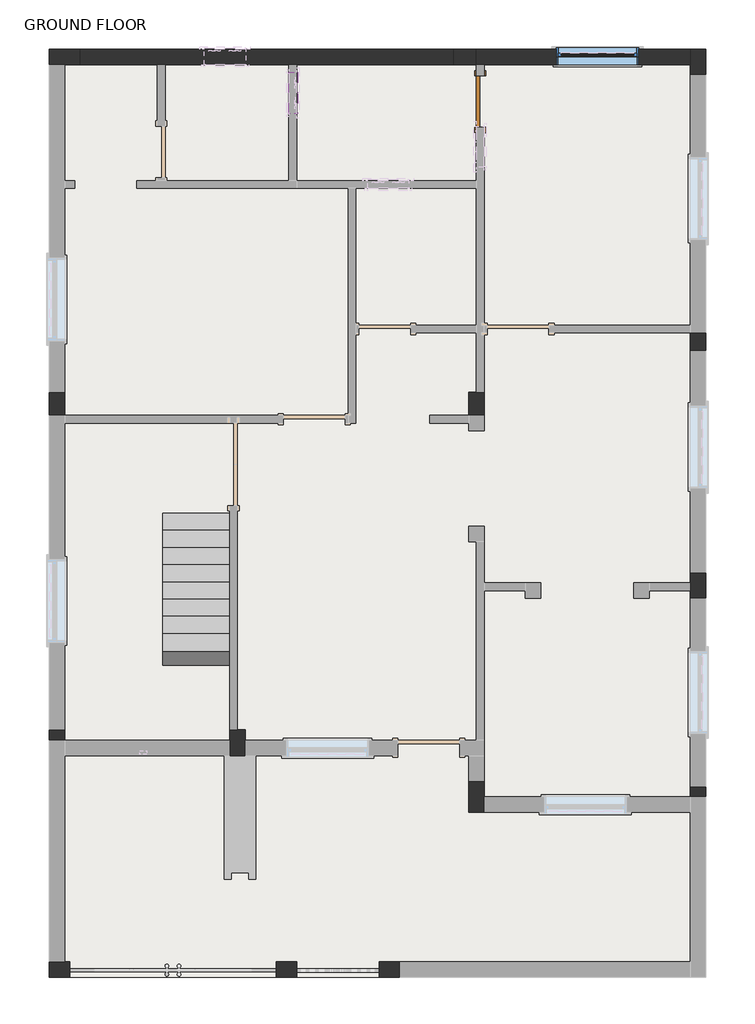
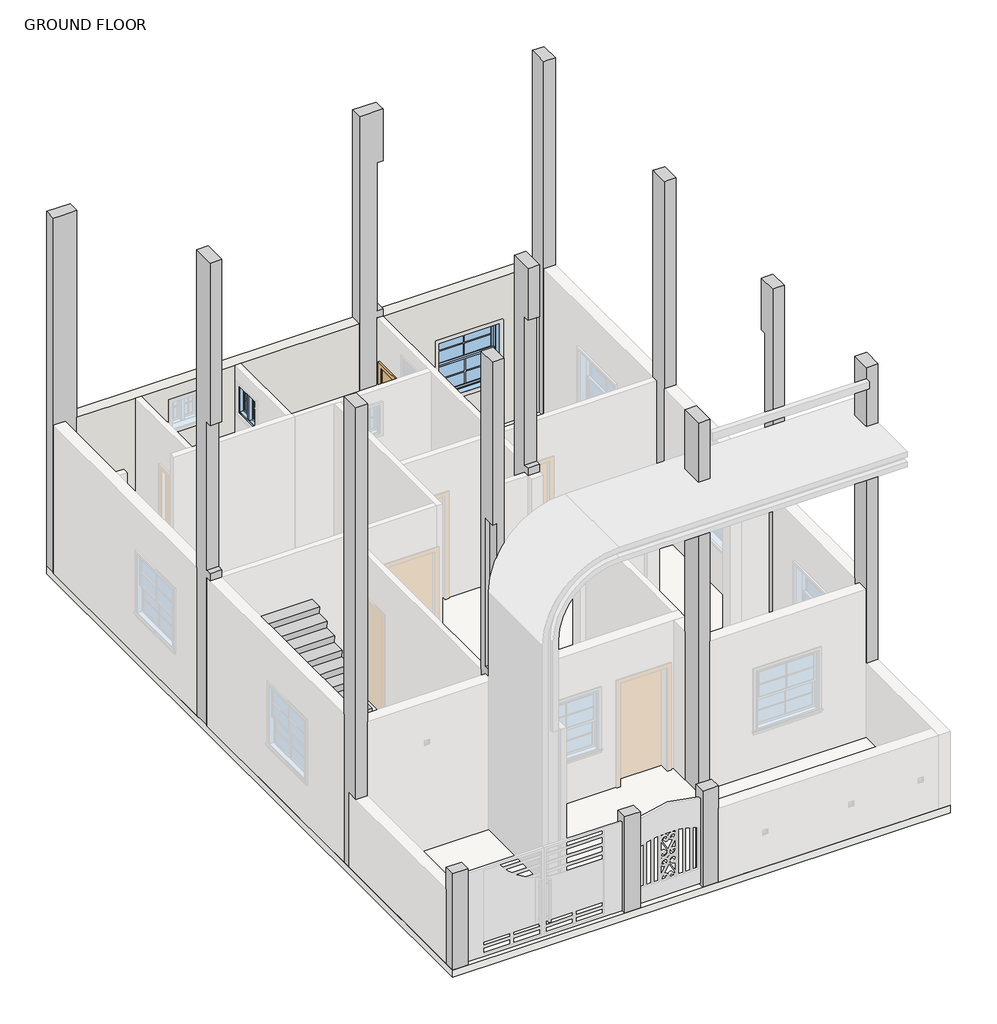
# One storey, part 2 of 3: 14 columns, 2 walls, 2 windows, 1 door, 1 slab, 1 stair flight.
"""IFC4 building model written with IfcOpenShell, lengths in millimetres."""

from ifc_helpers import new_model, si_unit, frame, origin, place, context, project, spatial, polyline, outline, extrude, faceted_brep, transform, mapped, element, save
from components import column_1646bf46, door_214872d5, window_casement_double_2_x2_e4709907, window_double_hung_4_x4_ec8efb0e

model = new_model("IFC4")

# Units and contexts
model_context = context("Model", 3, world=origin())
ifc_project = project(units=[si_unit("LENGTHUNIT", "METRE", prefix="MILLI")], contexts=[model_context])

# Site, building, storey
site = spatial("IfcSite", under=ifc_project)
building = spatial("IfcBuilding", under=site)
storey = spatial("IfcBuildingStorey", under=building, Name="GROUND FLOOR", Elevation=0.0)

# Columns
placement = place(None, origin())
element("IfcColumn", 1, ObjectType="Rectangular Column : 1'3\"X9\"", at=placement, inside=storey, context=model_context, shape_type="Brep", body=[
    faceted_brep([(-3417.2209734, 8887.7170657, 0.0), (-3188.6209734, 8887.7170657, 0.0), (-3188.6209734, 8506.7170657, 0.0), (-3417.2209734, 8506.7170657, 0.0), (-3417.2209734, 8659.1170657, 0.0), (-3417.2209734, 8887.7170657, 7315.2), (-3188.6209734, 8887.7170657, 7315.2), (-3417.2209734, 8887.7170657, 3048.0), (-3417.2209734, 8887.7170657, 3200.4), (-3417.2209734, 8887.7170657, 6248.4), (-3417.2209734, 8887.7170657, 6400.8), (-3188.6209734, 8506.7170657, 7315.2), (-3188.6209734, 8506.7170657, 6400.8), (-3188.6209734, 8506.7170657, 6248.4), (-3188.6209734, 8506.7170657, 3200.4), (-3188.6209734, 8506.7170657, 3048.0), (-3341.0209734, 8506.7170657, 7315.2), (-3417.2209734, 8506.7170657, 7315.2), (-3417.2209734, 8506.7170657, 6248.4), (-3417.2209734, 8506.7170657, 3200.4), (-3417.2209734, 8506.7170657, 3048.0), (-3417.2209734, 8735.3170657, 7315.2)], [[[0, 1, 2, 3, 4]], [[5, 6, 1, 0, 7, 8, 9, 10]], [[6, 11, 12, 13, 14, 15, 2, 1]], [[11, 16, 17, 18, 19, 20, 3, 2, 15, 14, 13, 12]], [[17, 21, 5, 10, 9, 8, 7, 0, 4, 3, 20, 19, 18]], [[5, 21, 17, 16, 11, 6]]]),
])
element("IfcColumn", 2, ObjectType="Rectangular Column : 1'3\"X9\"", at=placement, inside=storey, context=model_context, shape_type="Brep", body=[
    faceted_brep([(-3188.6209734, 4430.0170657, 0.0), (-3417.2209734, 4430.0170657, 0.0), (-3417.2209734, 4696.7170657, 0.0), (-3188.6209734, 4696.7170657, 0.0), (-3417.2209734, 4811.0170657, 7315.2), (-3341.0209734, 4811.0170657, 7315.2), (-3188.6209734, 4811.0170657, 7315.2), (-3188.6209734, 4811.0170657, 6400.8), (-3188.6209734, 4811.0170657, 6248.4), (-3188.6209734, 4811.0170657, 3200.4), (-3188.6209734, 4811.0170657, 3048.0), (-3417.2209734, 4811.0170657, 3048.0), (-3417.2209734, 4811.0170657, 3200.4), (-3417.2209734, 4811.0170657, 6248.4), (-3188.6209734, 4430.0170657, 7315.2), (-3188.6209734, 4430.0170657, 6400.8), (-3188.6209734, 4430.0170657, 6248.4), (-3188.6209734, 4430.0170657, 3200.4), (-3188.6209734, 4430.0170657, 3048.0), (-3188.6209734, 4696.7170657, 3048.0), (-3341.0209734, 4430.0170657, 7315.2), (-3417.2209734, 4430.0170657, 7315.2), (-3417.2209734, 4430.0170657, 6248.4), (-3417.2209734, 4430.0170657, 3200.4), (-3417.2209734, 4430.0170657, 3048.0), (-3417.2209734, 4696.7170657, 3048.0)], [[[0, 1, 2, 3]], [[4, 5, 6, 7, 8, 9, 10, 11, 12, 13]], [[6, 14, 15, 16, 17, 18, 0, 3, 19, 10, 9, 8, 7]], [[1, 0, 18, 17, 16, 15, 14, 20, 21, 22, 23, 24]], [[1, 24, 23, 22, 21, 4, 13, 12, 11, 25, 2]], [[6, 5, 4, 21, 20, 14]], [[19, 25, 11, 10]], [[25, 19, 3, 2]]]),
])
element("IfcColumn", 3, ObjectType="Rectangular Column : 1'3\"X9\"", at=placement, inside=storey, context=model_context, shape_type="Brep", body=[
    faceted_brep([(-3417.2209734, 1153.4170657, 0.0), (-3188.6209734, 1153.4170657, 0.0), (-3188.6209734, 772.4170657, 0.0), (-3417.2209734, 772.4170657, 0.0), (-3417.2209734, 886.7170657, 0.0), (-3417.2209734, 1001.0170657, 0.0), (-3417.2209734, 1153.4170657, 7315.2), (-3341.0209734, 1153.4170657, 7315.2), (-3188.6209734, 1153.4170657, 7315.2), (-3188.6209734, 1153.4170657, 6400.8), (-3188.6209734, 1153.4170657, 6248.4), (-3417.2209734, 1153.4170657, 6248.4), (-3188.6209734, 1153.4170657, 3048.0), (-3188.6209734, 1153.4170657, 3200.4), (-3188.6209734, 1039.1170657, 3200.4), (-3188.6209734, 1039.1170657, 6248.4), (-3188.6209734, 772.4170657, 7315.2), (-3188.6209734, 772.4170657, 6400.8), (-3188.6209734, 772.4170657, 6248.4), (-3188.6209734, 772.4170657, 3200.4), (-3188.6209734, 772.4170657, 3048.0), (-3341.0209734, 772.4170657, 7315.2), (-3417.2209734, 772.4170657, 7315.2), (-3417.2209734, 772.4170657, 6248.4), (-3417.2209734, 772.4170657, 3200.4), (-3417.2209734, 772.4170657, 3048.0), (-3417.2209734, 1039.1170657, 6248.4), (-3417.2209734, 1039.1170657, 3200.4), (-3417.2209734, 1153.4170657, 3200.4), (-3417.2209734, 1153.4170657, 3048.0)], [[[0, 1, 2, 3, 4, 5]], [[6, 7, 8, 9, 10, 11]], [[2, 1, 12, 13, 14, 15, 10, 9, 8, 16, 17, 18, 19, 20]], [[3, 2, 20, 19, 18, 17, 16, 21, 22, 23, 24, 25]], [[0, 5, 4, 3, 25, 24, 23, 22, 6, 11, 26, 27, 28, 29]], [[8, 7, 6, 22, 21, 16]], [[27, 14, 13, 28]], [[15, 26, 11, 10]], [[14, 27, 26, 15]], [[1, 0, 29, 28, 13, 12]]]),
])
element("IfcColumn", 4, ObjectType="Rectangular Column : 1'3\"X9\"", at=placement, inside=storey, context=model_context, shape_type="Brep", body=[
    faceted_brep([(-3417.2209734, -2008.8829343, 0.0), (-3188.6209734, -2008.8829343, 0.0), (-3188.6209734, -2161.2829343, 0.0), (-3417.2209734, -2161.2829343, 0.0), (-3417.2209734, -2008.8829343, 3048.0), (-3417.2209734, -2008.8829343, 3200.4), (-3417.2209734, -2008.8829343, 6248.4), (-3417.2209734, -2008.8829343, 7620.0), (-3188.6209734, -2008.8829343, 7620.0), (-3188.6209734, -2008.8829343, 7315.2), (-3188.6209734, -2008.8829343, 6400.8), (-3188.6209734, -2008.8829343, 6248.4), (-3188.6209734, -2008.8829343, 3200.4), (-3188.6209734, -2008.8829343, 3048.0), (-3188.6209734, -2389.8829343, 7620.0), (-3188.6209734, -2389.8829343, 3810.0), (-3188.6209734, -2389.8829343, 3200.4), (-3188.6209734, -2389.8829343, 1524.0), (-3188.6209734, -2161.2829343, 1524.0), (-3417.2209734, -2389.8829343, 7620.0), (-3417.2209734, -2389.8829343, 7315.2), (-3417.2209734, -2389.8829343, 6400.8), (-3417.2209734, -2389.8829343, 6248.4), (-3417.2209734, -2389.8829343, 3200.4), (-3417.2209734, -2389.8829343, 3048.0), (-3417.2209734, -2389.8829343, 1524.0), (-3417.2209734, -2161.2829343, 1524.0)], [[[0, 1, 2, 3]], [[1, 0, 4, 5, 6, 7, 8, 9, 10, 11, 12, 13]], [[1, 13, 12, 11, 10, 9, 8, 14, 15, 16, 17, 18, 2]], [[14, 19, 20, 21, 22, 23, 24, 25, 17, 16, 15]], [[7, 6, 5, 4, 0, 3, 26, 25, 24, 23, 22, 21, 20, 19]], [[8, 7, 19, 14]], [[26, 18, 17, 25]], [[18, 26, 3, 2]]]),
])
element("IfcColumn", 5, ObjectType="Rectangular Column : 1'3\"X9\"", at=placement, inside=storey, context=model_context, shape_type="Brep", body=[
    faceted_brep([(-10224.4209734, -1170.6829343, 0.0), (-10110.1209734, -1170.6829343, 0.0), (-9995.8209734, -1170.6829343, 0.0), (-9995.8209734, -1323.0829343, 0.0), (-9995.8209734, -1551.6829343, 0.0), (-10224.4209734, -1551.6829343, 0.0), (-10224.4209734, -1323.0829343, 0.0), (-10224.4209734, -1170.6829343, 3048.0), (-10224.4209734, -1170.6829343, 3200.4), (-10224.4209734, -1170.6829343, 6248.4), (-10224.4209734, -1170.6829343, 6400.8), (-10224.4209734, -1170.6829343, 9448.8), (-10224.4209734, -1170.6829343, 9601.2), (-9995.8209734, -1170.6829343, 9601.2), (-9995.8209734, -1170.6829343, 9448.8), (-9995.8209734, -1170.6829343, 6400.8), (-9995.8209734, -1551.6829343, 9601.2), (-9995.8209734, -1551.6829343, 7315.2), (-9995.8209734, -1551.6829343, 6400.8), (-9995.8209734, -1551.6829343, 6248.4), (-9995.8209734, -1551.6829343, 3200.4), (-9995.8209734, -1551.6829343, 3048.0), (-10224.4209734, -1551.6829343, 9601.2), (-10224.4209734, -1551.6829343, 9448.8), (-10224.4209734, -1551.6829343, 6400.8), (-10224.4209734, -1551.6829343, 6248.4), (-10148.2209734, -1551.6829343, 6248.4), (-10148.2209734, -1551.6829343, 3200.4), (-10224.4209734, -1551.6829343, 3200.4), (-10224.4209734, -1551.6829343, 3048.0), (-10224.4209734, -1323.0829343, 3200.4), (-10224.4209734, -1323.0829343, 6248.4), (-10148.2209734, -1323.0829343, 3200.4), (-10148.2209734, -1323.0829343, 6248.4)], [[[0, 1, 2, 3, 4, 5, 6]], [[2, 1, 0, 7, 8, 9, 10, 11, 12, 13, 14, 15]], [[4, 3, 2, 15, 14, 13, 16, 17, 18, 19, 20, 21]], [[5, 4, 21, 20, 19, 18, 17, 16, 22, 23, 24, 25, 26, 27, 28, 29]], [[0, 6, 5, 29, 28, 30, 31, 25, 24, 23, 22, 12, 11, 10, 9, 8, 7]], [[13, 12, 22, 16]], [[32, 33, 31, 30]], [[27, 32, 30, 28]], [[33, 26, 25, 31]], [[33, 32, 27, 26]]]),
])
element("IfcColumn", 6, ObjectType="Rectangular Column : 1'3\"X9\"", at=placement, inside=storey, context=model_context, shape_type="Brep", body=[
    faceted_brep([(-12891.4209734, -1170.6829343, 0.0), (-12662.8209734, -1170.6829343, 0.0), (-12662.8209734, -1323.0829343, 0.0), (-12891.4209734, -1323.0829343, 0.0), (-12891.4209734, -1170.6829343, 3048.0), (-12891.4209734, -1170.6829343, 3200.4), (-12891.4209734, -1170.6829343, 6248.4), (-12891.4209734, -1170.6829343, 6400.8), (-12891.4209734, -1170.6829343, 9448.8), (-12891.4209734, -1170.6829343, 9601.2), (-12662.8209734, -1170.6829343, 9601.2), (-12662.8209734, -1170.6829343, 9448.8), (-12662.8209734, -1170.6829343, 6400.8), (-12662.8209734, -1170.6829343, 6248.4), (-12662.8209734, -1170.6829343, 3200.4), (-12662.8209734, -1170.6829343, 3048.0), (-12662.8209734, -1551.6829343, 9601.2), (-12662.8209734, -1551.6829343, 9448.8), (-12662.8209734, -1551.6829343, 6400.8), (-12662.8209734, -1551.6829343, 6248.4), (-12662.8209734, -1551.6829343, 3200.4), (-12662.8209734, -1551.6829343, 3048.0), (-12662.8209734, -1551.6829343, 1524.0), (-12662.8209734, -1323.0829343, 1524.0), (-12891.4209734, -1551.6829343, 9601.2), (-12891.4209734, -1551.6829343, 1524.0), (-12891.4209734, -1323.0829343, 1524.0)], [[[0, 1, 2, 3]], [[1, 0, 4, 5, 6, 7, 8, 9, 10, 11, 12, 13, 14, 15]], [[1, 15, 14, 13, 12, 11, 10, 16, 17, 18, 19, 20, 21, 22, 23, 2]], [[16, 24, 25, 22, 21, 20, 19, 18, 17]], [[9, 8, 7, 6, 5, 4, 0, 3, 26, 25, 24]], [[10, 9, 24, 16]], [[26, 23, 22, 25]], [[23, 26, 3, 2]]]),
])
element("IfcColumn", 7, ObjectType="Rectangular Column : 1'6\"X9\"", at=placement, inside=storey, context=model_context, shape_type="Brep", body=[
    faceted_brep([(-12434.2209734, 8887.7170657, 0.0), (-12434.2209734, 8659.1170657, 0.0), (-12662.8209734, 8659.1170657, 0.0), (-12891.4209734, 8659.1170657, 0.0), (-12891.4209734, 8887.7170657, 0.0), (-12434.2209734, 8887.7170657, 7315.2), (-12434.2209734, 8735.3170657, 7315.2), (-12434.2209734, 8659.1170657, 7315.2), (-12434.2209734, 8659.1170657, 6248.4), (-12434.2209734, 8659.1170657, 3200.4), (-12434.2209734, 8659.1170657, 3048.0), (-12434.2209734, 8887.7170657, 3048.0), (-12434.2209734, 8887.7170657, 3200.4), (-12434.2209734, 8887.7170657, 6248.4), (-12434.2209734, 8887.7170657, 6400.8), (-12739.0209734, 8659.1170657, 7315.2), (-12891.4209734, 8659.1170657, 7315.2), (-12891.4209734, 8659.1170657, 6400.8), (-12891.4209734, 8659.1170657, 6248.4), (-12891.4209734, 8659.1170657, 3200.4), (-12891.4209734, 8659.1170657, 3048.0), (-12891.4209734, 8887.7170657, 7315.2)], [[[0, 1, 2, 3, 4]], [[5, 6, 7, 8, 9, 10, 1, 0, 11, 12, 13, 14]], [[7, 15, 16, 17, 18, 19, 20, 3, 2, 1, 10, 9, 8]], [[16, 21, 4, 3, 20, 19, 18, 17]], [[21, 5, 14, 13, 12, 11, 0, 4]], [[5, 21, 16, 15, 7, 6]]]),
])
element("IfcColumn", 8, ObjectType="Rectangular Column : 1'6\"X9\"", at=placement, inside=storey, context=model_context, shape_type="Brep", body=[
    faceted_brep([(-6922.4209734, 8659.1170657, 0.0), (-6922.4209734, 8887.7170657, 0.0), (-6579.5209734, 8887.7170657, 0.0), (-6579.5209734, 8659.1170657, 0.0), (-6465.2209734, 8887.7170657, 7315.2), (-6465.2209734, 8735.3170657, 7315.2), (-6465.2209734, 8659.1170657, 7315.2), (-6465.2209734, 8659.1170657, 6248.4), (-6465.2209734, 8887.7170657, 6248.4), (-6465.2209734, 8887.7170657, 6400.8), (-6922.4209734, 8659.1170657, 7315.2), (-6922.4209734, 8659.1170657, 6248.4), (-6922.4209734, 8659.1170657, 3200.4), (-6922.4209734, 8659.1170657, 3048.0), (-6579.5209734, 8659.1170657, 3048.0), (-6465.2209734, 8659.1170657, 3048.0), (-6465.2209734, 8659.1170657, 3200.4), (-6579.5209734, 8659.1170657, 3200.4), (-6579.5209734, 8659.1170657, 6248.4), (-6922.4209734, 8735.3170657, 7315.2), (-6922.4209734, 8887.7170657, 7315.2), (-6922.4209734, 8887.7170657, 6400.8), (-6922.4209734, 8887.7170657, 6248.4), (-6922.4209734, 8887.7170657, 3200.4), (-6922.4209734, 8887.7170657, 3048.0), (-6579.5209734, 8887.7170657, 6248.4), (-6579.5209734, 8887.7170657, 3200.4), (-6465.2209734, 8887.7170657, 3200.4), (-6465.2209734, 8887.7170657, 3048.0), (-6579.5209734, 8887.7170657, 3048.0)], [[[0, 1, 2, 3]], [[4, 5, 6, 7, 8, 9]], [[6, 10, 11, 12, 13, 0, 3, 14, 15, 16, 17, 18, 7]], [[1, 0, 13, 12, 11, 10, 19, 20, 21, 22, 23, 24]], [[1, 24, 23, 22, 21, 20, 4, 9, 8, 25, 26, 27, 28, 29, 2]], [[6, 5, 4, 20, 19, 10]], [[14, 29, 28, 15]], [[29, 14, 3, 2]], [[26, 17, 16, 27]], [[18, 25, 8, 7]], [[17, 26, 25, 18]], [[15, 28, 27, 16]]]),
])
element("IfcColumn", 9, ObjectType="Rectangular Column : 1'6\"X9\"", at=placement, inside=storey, context=model_context, shape_type="Brep", body=[
    faceted_brep([(-12891.4209734, 3820.4170657, 0.0), (-12662.8209734, 3820.4170657, 0.0), (-12662.8209734, 3477.5170657, 0.0), (-12891.4209734, 3477.5170657, 0.0), (-12891.4209734, 3820.4170657, 3048.0), (-12891.4209734, 3820.4170657, 3200.4), (-12891.4209734, 3820.4170657, 6248.4), (-12891.4209734, 3820.4170657, 6400.8), (-12891.4209734, 3820.4170657, 7315.2), (-12891.4209734, 3820.4170657, 9601.2), (-12662.8209734, 3820.4170657, 9601.2), (-12662.8209734, 3820.4170657, 9448.8), (-12662.8209734, 3820.4170657, 6400.8), (-12662.8209734, 3820.4170657, 6248.4), (-12662.8209734, 3820.4170657, 3200.4), (-12662.8209734, 3820.4170657, 3048.0), (-12662.8209734, 3363.2170657, 9601.2), (-12662.8209734, 3363.2170657, 9448.8), (-12662.8209734, 3363.2170657, 6400.8), (-12662.8209734, 3363.2170657, 6248.4), (-12662.8209734, 3477.5170657, 6248.4), (-12662.8209734, 3477.5170657, 3200.4), (-12662.8209734, 3363.2170657, 3200.4), (-12662.8209734, 3363.2170657, 3048.0), (-12662.8209734, 3477.5170657, 3048.0), (-12891.4209734, 3363.2170657, 9601.2), (-12891.4209734, 3363.2170657, 9448.8), (-12891.4209734, 3363.2170657, 6400.8), (-12891.4209734, 3363.2170657, 6248.4), (-12891.4209734, 3477.5170657, 3048.0), (-12891.4209734, 3363.2170657, 3048.0), (-12891.4209734, 3363.2170657, 3200.4), (-12891.4209734, 3477.5170657, 3200.4), (-12891.4209734, 3477.5170657, 6248.4)], [[[0, 1, 2, 3]], [[1, 0, 4, 5, 6, 7, 8, 9, 10, 11, 12, 13, 14, 15]], [[1, 15, 14, 13, 12, 11, 10, 16, 17, 18, 19, 20, 21, 22, 23, 24, 2]], [[16, 25, 26, 27, 28, 19, 18, 17]], [[9, 8, 7, 6, 5, 4, 0, 3, 29, 30, 31, 32, 33, 28, 27, 26, 25]], [[10, 9, 25, 16]], [[29, 24, 23, 30]], [[24, 29, 3, 2]], [[21, 32, 31, 22]], [[33, 20, 19, 28]], [[32, 21, 20, 33]], [[30, 23, 22, 31]]]),
])
element("IfcColumn", 10, ObjectType="Rectangular Column : 1'6\"X9\"", at=placement, inside=storey, context=model_context, shape_type="Brep", body=[
    faceted_brep([(-6693.8209734, 3820.4170657, 0.0), (-6579.5209734, 3820.4170657, 0.0), (-6465.2209734, 3820.4170657, 0.0), (-6465.2209734, 3477.5170657, 0.0), (-6693.8209734, 3477.5170657, 0.0), (-6693.8209734, 3820.4170657, 7315.2), (-6465.2209734, 3820.4170657, 7315.2), (-6465.2209734, 3820.4170657, 6248.4), (-6465.2209734, 3820.4170657, 3200.4), (-6465.2209734, 3820.4170657, 3048.0), (-6465.2209734, 3363.2170657, 7315.2), (-6465.2209734, 3363.2170657, 6248.4), (-6465.2209734, 3477.5170657, 6248.4), (-6465.2209734, 3477.5170657, 3200.4), (-6465.2209734, 3363.2170657, 3200.4), (-6465.2209734, 3363.2170657, 3048.0), (-6465.2209734, 3477.5170657, 3048.0), (-6693.8209734, 3363.2170657, 7315.2), (-6693.8209734, 3363.2170657, 6248.4), (-6693.8209734, 3477.5170657, 3048.0), (-6693.8209734, 3363.2170657, 3048.0), (-6693.8209734, 3363.2170657, 3200.4), (-6693.8209734, 3477.5170657, 3200.4), (-6693.8209734, 3477.5170657, 6248.4)], [[[0, 1, 2, 3, 4]], [[2, 1, 0, 5, 6, 7, 8, 9]], [[2, 9, 8, 7, 6, 10, 11, 12, 13, 14, 15, 16, 3]], [[10, 17, 18, 11]], [[5, 0, 4, 19, 20, 21, 22, 23, 18, 17]], [[6, 5, 17, 10]], [[19, 16, 15, 20]], [[16, 19, 4, 3]], [[13, 22, 21, 14]], [[23, 12, 11, 18]], [[22, 13, 12, 23]], [[20, 15, 14, 21]]]),
])
element("IfcColumn", 11, ObjectType="Rectangular Column : 1'6\"X9\"", at=placement, inside=storey, context=model_context, shape_type="Brep", body=[
    faceted_brep([(-6693.8209734, -1932.6829343, 0.0), (-6465.2209734, -1932.6829343, 0.0), (-6465.2209734, -2161.2829343, 0.0), (-6465.2209734, -2389.8829343, 0.0), (-6693.8209734, -2389.8829343, 0.0), (-6693.8209734, -1932.6829343, 7620.0), (-6465.2209734, -1932.6829343, 7620.0), (-6465.2209734, -1932.6829343, 6248.4), (-6465.2209734, -1932.6829343, 3200.4), (-6465.2209734, -1932.6829343, 3048.0), (-6693.8209734, -1932.6829343, 3048.0), (-6693.8209734, -1932.6829343, 3200.4), (-6693.8209734, -1932.6829343, 6248.4), (-6693.8209734, -1932.6829343, 6400.8), (-6693.8209734, -1932.6829343, 7315.2), (-6465.2209734, -2389.8829343, 7620.0), (-6465.2209734, -2389.8829343, 7315.2), (-6465.2209734, -2389.8829343, 6400.8), (-6465.2209734, -2389.8829343, 6248.4), (-6465.2209734, -2389.8829343, 3200.4), (-6465.2209734, -2389.8829343, 3048.0), (-6693.8209734, -2389.8829343, 7620.0)], [[[0, 1, 2, 3, 4]], [[5, 6, 7, 8, 9, 1, 0, 10, 11, 12, 13, 14]], [[6, 15, 16, 17, 18, 19, 20, 3, 2, 1, 9, 8, 7]], [[15, 21, 4, 3, 20, 19, 18, 17, 16]], [[21, 5, 14, 13, 12, 11, 10, 0, 4]], [[5, 21, 15, 6]]]),
])
element("IfcColumn", 12, ObjectType="Rectangular Column : 1'X9\"", at=placement, inside=storey, context=model_context, shape_type="Brep", body=[
    faceted_brep([(-12586.6209734, -4599.6829343, 0.0), (-12586.6209734, -4828.2829343, 0.0), (-12891.4209734, -4828.2829343, 0.0), (-12891.4209734, -4599.6829343, 0.0), (-12662.8209734, -4599.6829343, 0.0), (-12586.6209734, -4599.6829343, 1981.2), (-12586.6209734, -4828.2829343, 1981.2), (-12891.4209734, -4828.2829343, 1981.2), (-12891.4209734, -4599.6829343, 1981.2), (-12891.4209734, -4599.6829343, 1524.0)], [[[0, 1, 2, 3, 4]], [[5, 6, 1, 0]], [[6, 7, 2, 1]], [[7, 8, 9, 3, 2]], [[8, 5, 0, 4, 3, 9]], [[5, 8, 7, 6]]]),
])
element("IfcColumn", 13, ObjectType="Rectangular Column : 1'X9\"", at=placement, inside=storey, context=model_context, shape_type="Brep", body=[
    faceted_brep([(-7709.8209734, -4599.6829343, 0.0), (-7709.8209734, -4828.2829343, 0.0), (-8014.6209734, -4828.2829343, 0.0), (-8014.6209734, -4599.6829343, 0.0), (-7709.8209734, -4599.6829343, 1981.2), (-7709.8209734, -4828.2829343, 1981.2), (-7709.8209734, -4828.2829343, 1524.0), (-7709.8209734, -4599.6829343, 1524.0), (-8014.6209734, -4828.2829343, 1981.2), (-8014.6209734, -4599.6829343, 1981.2)], [[[0, 1, 2, 3]], [[4, 5, 6, 1, 0, 7]], [[5, 8, 2, 1, 6]], [[8, 9, 3, 2]], [[9, 4, 7, 0, 3]], [[4, 9, 8, 5]]]),
])
column_shape = column_1646bf46(model_context)
element("IfcColumn", 14, ObjectType="Rectangular Column : 1'X9\"", at=placement, inside=storey, context=model_context, shape_type="MappedRepresentation", body=[
    mapped(column_shape, transform((-9386.2209734, -4713.9829343, 0.0), x_axis=(1.0, 0.0, 0.0), y_axis=(0.0, 1.0, 0.0), z_axis=(0.0, 0.0, 1.0))),
])

# Door
door_shape = door_214872d5(model_context)
element("IfcDoor", 15, ObjectType="Single-Flush : 2'6\"", at=placement, inside=storey, context=model_context, shape_type="MappedRepresentation", body=[
    mapped(door_shape, transform((-6522.3709734, 8113.0170657, 0.0), x_axis=(0.0, 1.0, 0.0), y_axis=(-1.0, 0.0, 0.0), z_axis=(0.0, 0.0, 1.0))),
])

# Slab
element("IfcSlab", 16, ObjectType="6\"", at=placement, inside=storey, context=model_context, shape_type="SweptSolid", body=[
    extrude(outline(polyline([(-3188.6209734, 8887.7170657), (-3188.6209734, -4828.2829343), (-12891.4209734, -4828.2829343), (-12891.4209734, 8887.7170657), (-3188.6209734, 8887.7170657)])), frame((0.0, 0.0, -152.4), z_axis=(0.0, 0.0, 1.0), x_axis=(1.0, 0.0, 0.0)), (0.0, 0.0, 1.0), 152.4),
])

# Stair flight
element("IfcStairFlight", 17, ObjectType="3/4\" Nosing", at=placement, inside=storey, context=model_context, shape_type="Brep", body=[
    faceted_brep([(-10224.4209734, 2029.7170657, 145.4727273), (-11215.0209735, 2029.7170657, 145.4727273), (-11215.0209735, 1756.6670657, 145.4727273), (-10224.4209734, 1756.6670657, 145.4727273), (-10224.4209734, 1756.6670657, 72.2955816), (-10224.4209734, 1882.8974463, 0.0), (-10224.4209734, 2010.6670657, 0.0), (-11215.0209735, 2010.6670657, 0.0), (-11215.0209735, 1882.8974463, 0.0), (-11215.0209735, 1756.6670657, 72.2955816), (-10224.4209734, 1775.7170657, 290.9454545), (-11215.0209735, 1775.7170657, 290.9454545), (-11215.0209735, 1502.6670657, 290.9454545), (-10224.4209734, 1502.6670657, 290.9454545), (-10224.4209734, 1502.6670657, 217.7683089), (-11215.0209735, 1502.6670657, 217.7683089), (-10224.4209734, 1521.7170657, 436.4181818), (-11215.0209735, 1521.7170657, 436.4181818), (-11215.0209735, 1248.6670657, 436.4181818), (-10224.4209734, 1248.6670657, 436.4181818), (-10224.4209734, 1248.6670657, 363.2410361), (-11215.0209735, 1248.6670657, 363.2410361), (-10224.4209734, 1267.7170657, 581.8909091), (-11215.0209735, 1267.7170657, 581.8909091), (-11215.0209735, 994.6670657, 581.8909091), (-10224.4209734, 994.6670657, 581.8909091), (-10224.4209734, 994.6670657, 508.7137634), (-11215.0209735, 994.6670657, 508.7137634), (-10224.4209734, 1013.7170657, 727.3636364), (-11215.0209735, 1013.7170657, 727.3636364), (-11215.0209735, 740.6670657, 727.3636364), (-10224.4209734, 740.6670657, 727.3636364), (-10224.4209734, 740.6670657, 654.1864907), (-11215.0209735, 740.6670657, 654.1864907), (-10224.4209734, 759.7170657, 872.8363636), (-11215.0209735, 759.7170657, 872.8363636), (-11215.0209735, 486.6670657, 872.8363636), (-10224.4209734, 486.6670657, 872.8363636), (-10224.4209734, 486.6670657, 799.659218), (-11215.0209735, 486.6670657, 799.659218), (-10224.4209734, 505.7170657, 1018.3090909), (-11215.0209735, 505.7170657, 1018.3090909), (-11215.0209735, 232.6670657, 1018.3090909), (-10224.4209734, 232.6670657, 1018.3090909), (-10224.4209734, 232.6670657, 945.1319452), (-11215.0209735, 232.6670657, 945.1319452), (-10224.4209734, 251.7170657, 1163.7818182), (-11215.0209735, 251.7170657, 1163.7818182), (-11215.0209735, -21.3329343, 1163.7818182), (-10224.4209734, -21.3329343, 1163.7818182), (-10224.4209734, -21.3329343, 1090.6046725), (-11215.0209735, -21.3329343, 1090.6046725), (-10224.4209734, -2.2829343, 1309.2545455), (-11215.0209735, -2.2829343, 1309.2545455), (-11215.0209735, -275.3329343, 1309.2545455), (-10224.4209734, -275.3329343, 1309.2545455), (-10224.4209734, -275.3329343, 1236.0773998), (-11215.0209735, -275.3329343, 1236.0773998), (-10224.4209734, -256.2829343, 1454.7272727), (-11215.0209735, -256.2829343, 1454.7272727), (-11215.0209735, -529.3329343, 1454.7272727), (-10224.4209734, -529.3329343, 1454.7272727), (-10224.4209734, -529.3329343, 1381.5501271), (-11215.0209735, -800.2295379, 1536.7), (-11215.0209735, -518.5984105, 1536.7), (-12662.8209734, -491.2329343, 1600.2), (-12662.8209734, -1323.0829343, 1600.2), (-10224.4209734, -1323.0829343, 1600.2), (-10224.4209734, -800.2295379, 1600.2), (-10224.4209734, -510.2829343, 1600.2), (-11215.0209735, -510.2829343, 1600.2), (-11672.2209734, -510.2829343, 1600.2), (-11672.2209734, -491.2329343, 1600.2), (-12662.8209734, -491.2329343, 1536.7), (-12662.8209734, -1323.0829343, 1536.7), (-10224.4209734, -1323.0829343, 1536.7), (-10224.4209734, -800.2295379, 1536.7), (-11215.0209735, -510.2829343, 1536.7), (-11672.2209734, -510.2829343, 1536.7), (-11672.2209734, -491.2329343, 1536.7), (-12662.8209734, -510.2829343, 1745.6727273), (-11672.2209734, -510.2829343, 1745.6727273), (-11672.2209734, -474.3363307, 1745.6727273), (-11672.2209734, -237.2329343, 1745.6727273), (-12662.8209734, -237.2329343, 1745.6727273), (-12662.8209734, -474.3363307, 1745.6727273), (-12662.8209734, -237.2329343, 1672.4955816), (-12662.8209734, -474.3363307, 1536.7), (-11672.2209734, -474.3363307, 1536.7), (-11672.2209734, -237.2329343, 1672.4955816), (-12662.8209734, -256.2829343, 1891.1454545), (-11672.2209734, -256.2829343, 1891.1454545), (-11672.2209734, 16.7670657, 1891.1454545), (-12662.8209734, 16.7670657, 1891.1454545), (-12662.8209734, 16.7670657, 1817.9683089), (-11672.2209734, 16.7670657, 1817.9683089), (-12662.8209734, -2.2829343, 2036.6181818), (-11672.2209734, -2.2829343, 2036.6181818), (-11672.2209734, 270.7670657, 2036.6181818), (-12662.8209734, 270.7670657, 2036.6181818), (-12662.8209734, 270.7670657, 1963.4410361), (-11672.2209734, 270.7670657, 1963.4410361), (-12662.8209734, 251.7170657, 2182.0909091), (-11672.2209734, 251.7170657, 2182.0909091), (-11672.2209734, 524.7670657, 2182.0909091), (-12662.8209734, 524.7670657, 2182.0909091), (-12662.8209734, 524.7670657, 2108.9137634), (-11672.2209734, 524.7670657, 2108.9137634), (-12662.8209734, 505.7170657, 2327.5636364), (-11672.2209734, 505.7170657, 2327.5636364), (-11672.2209734, 778.7670657, 2327.5636364), (-12662.8209734, 778.7670657, 2327.5636364), (-12662.8209734, 778.7670657, 2254.3864907), (-11672.2209734, 778.7670657, 2254.3864907), (-12662.8209734, 759.7170657, 2473.0363636), (-11672.2209734, 759.7170657, 2473.0363636), (-11672.2209734, 1032.7670657, 2473.0363636), (-12662.8209734, 1032.7670657, 2473.0363636), (-12662.8209734, 1032.7670657, 2399.859218), (-11672.2209734, 1032.7670657, 2399.859218), (-12662.8209734, 1013.7170657, 2618.5090909), (-11672.2209734, 1013.7170657, 2618.5090909), (-11672.2209734, 1286.7670657, 2618.5090909), (-12662.8209734, 1286.7670657, 2618.5090909), (-12662.8209734, 1286.7670657, 2545.3319452), (-11672.2209734, 1286.7670657, 2545.3319452), (-12662.8209734, 1267.7170657, 2763.9818182), (-11672.2209734, 1267.7170657, 2763.9818182), (-11672.2209734, 1540.7670657, 2763.9818182), (-12662.8209734, 1540.7670657, 2763.9818182), (-12662.8209734, 1540.7670657, 2690.8046725), (-11672.2209734, 1540.7670657, 2690.8046725), (-12662.8209734, 1521.7170657, 2909.4545455), (-11672.2209734, 1521.7170657, 2909.4545455), (-11672.2209734, 1794.7670657, 2909.4545455), (-12662.8209734, 1794.7670657, 2909.4545455), (-12662.8209734, 1794.7670657, 2836.2773998), (-11672.2209734, 1794.7670657, 2836.2773998), (-12662.8209734, 1775.7170657, 3054.9272727), (-11672.2209734, 1775.7170657, 3054.9272727), (-11672.2209734, 2029.7170657, 3054.9272727), (-12662.8209734, 2029.7170657, 3054.9272727), (-12662.8209734, 2029.7170657, 2970.8396725), (-11672.2209734, 2029.7170657, 2970.8396725)], [[[0, 1, 2, 3]], [[0, 3, 4, 5, 6]], [[2, 1, 7, 8, 9]], [[10, 11, 12, 13]], [[10, 13, 14, 4, 3]], [[12, 11, 2, 9, 15]], [[16, 17, 18, 19]], [[16, 19, 20, 14, 13]], [[18, 17, 12, 15, 21]], [[22, 23, 24, 25]], [[22, 25, 26, 20, 19]], [[24, 23, 18, 21, 27]], [[28, 29, 30, 31]], [[28, 31, 32, 26, 25]], [[30, 29, 24, 27, 33]], [[34, 35, 36, 37]], [[34, 37, 38, 32, 31]], [[36, 35, 30, 33, 39]], [[40, 41, 42, 43]], [[40, 43, 44, 38, 37]], [[42, 41, 36, 39, 45]], [[46, 47, 48, 49]], [[46, 49, 50, 44, 43]], [[48, 47, 42, 45, 51]], [[52, 53, 54, 55]], [[52, 55, 56, 50, 49]], [[54, 53, 48, 51, 57]], [[58, 59, 60, 61]], [[58, 61, 62, 56, 55]], [[59, 54, 57, 63, 64, 60]], [[65, 66, 67, 68, 69, 70, 71, 72]], [[66, 65, 73, 74]], [[67, 66, 74, 75]], [[61, 69, 68, 67, 75, 76, 62]], [[70, 64, 77]], [[71, 70, 77, 78]], [[72, 71, 78, 79]], [[80, 81, 82, 83, 84, 85]], [[65, 80, 85, 84, 86, 87, 73]], [[81, 72, 79, 88, 89, 83, 82]], [[90, 91, 92, 93]], [[90, 93, 94, 86, 84]], [[92, 91, 83, 89, 95]], [[96, 97, 98, 99]], [[96, 99, 100, 94, 93]], [[98, 97, 92, 95, 101]], [[102, 103, 104, 105]], [[102, 105, 106, 100, 99]], [[104, 103, 98, 101, 107]], [[108, 109, 110, 111]], [[108, 111, 112, 106, 105]], [[110, 109, 104, 107, 113]], [[114, 115, 116, 117]], [[114, 117, 118, 112, 111]], [[116, 115, 110, 113, 119]], [[120, 121, 122, 123]], [[120, 123, 124, 118, 117]], [[122, 121, 116, 119, 125]], [[126, 127, 128, 129]], [[126, 129, 130, 124, 123]], [[128, 127, 122, 125, 131]], [[132, 133, 134, 135]], [[132, 135, 136, 130, 129]], [[134, 133, 128, 131, 137]], [[1, 0, 6, 7]], [[3, 2, 11, 10]], [[13, 12, 17, 16]], [[19, 18, 23, 22]], [[25, 24, 29, 28]], [[31, 30, 35, 34]], [[37, 36, 41, 40]], [[43, 42, 47, 46]], [[49, 48, 53, 52]], [[55, 54, 59, 58]], [[61, 60, 64, 70, 69]], [[65, 72, 81, 80]], [[84, 83, 91, 90]], [[93, 92, 97, 96]], [[99, 98, 103, 102]], [[105, 104, 109, 108]], [[111, 110, 115, 114]], [[117, 116, 121, 120]], [[123, 122, 127, 126]], [[129, 128, 133, 132]], [[138, 139, 140, 141]], [[138, 141, 142, 136, 135]], [[140, 139, 134, 137, 143]], [[141, 140, 143, 142]], [[135, 134, 139, 138]], [[7, 6, 5, 8]], [[76, 63, 57, 51, 45, 39, 33, 27, 21, 15, 9, 8, 5, 4, 14, 20, 26, 32, 38, 44, 50, 56, 62]], [[63, 76, 75, 74, 73, 87, 88, 79, 78, 77, 64]], [[88, 87, 86, 94, 100, 106, 112, 118, 124, 130, 136, 142, 143, 137, 131, 125, 119, 113, 107, 101, 95, 89]]]),
])

# Walls
element("IfcWall", 18, ObjectType="9\"", at=placement, inside=storey, context=model_context, shape_type="Brep", body=[
    faceted_brep([(-12434.2209734, 8659.1170657, 0.0), (-11291.2209734, 8659.1170657, 0.0), (-11176.9209734, 8659.1170657, 0.0), (-9348.1209734, 8659.1170657, 0.0), (-9233.8209734, 8659.1170657, 0.0), (-6922.4209734, 8659.1170657, 0.0), (-6922.4209734, 8659.1170657, 3048.0), (-9233.8209734, 8659.1170657, 3048.0), (-9348.1209734, 8659.1170657, 3048.0), (-11176.9209734, 8659.1170657, 3048.0), (-11291.2209734, 8659.1170657, 3048.0), (-12434.2209734, 8659.1170657, 3048.0), (-9989.4709734, 8659.1170657, 2743.2), (-9989.4709734, 8659.1170657, 2133.6), (-10599.0709734, 8659.1170657, 2133.6), (-10599.0709734, 8659.1170657, 2743.2), (-12434.2209734, 8887.7170657, 0.0), (-12434.2209734, 8887.7170657, 3048.0), (-6922.4209734, 8887.7170657, 3048.0), (-6922.4209734, 8887.7170657, 0.0), (-9989.4709734, 8887.7170657, 2743.2), (-10599.0709734, 8887.7170657, 2743.2), (-10599.0709734, 8887.7170657, 2133.6), (-9989.4709734, 8887.7170657, 2133.6)], [[[0, 1, 2, 3, 4, 5, 6, 7, 8, 9, 10, 11], [12, 13, 14, 15]], [[16, 17, 18, 19], [20, 21, 22, 23]], [[5, 4, 3, 2, 1, 0, 16, 19]], [[6, 5, 19, 18]], [[11, 10, 9, 8, 7, 6, 18, 17]], [[0, 11, 17, 16]], [[13, 12, 20, 23]], [[14, 13, 23, 22]], [[15, 14, 22, 21]], [[12, 15, 21, 20]]]),
])
element("IfcWall", 19, ObjectType="9\"", at=placement, inside=storey, context=model_context, shape_type="Brep", body=[
    faceted_brep([(-6579.5209734, 8659.1170657, 0.0), (-6465.2209734, 8659.1170657, 0.0), (-3417.2209734, 8659.1170657, 0.0), (-3417.2209734, 8659.1170657, 3048.0), (-6465.2209734, 8659.1170657, 3048.0), (-6579.5209734, 8659.1170657, 3048.0), (-5398.4209734, 8659.1170657, 2133.6), (-4179.2209734, 8659.1170657, 2133.6), (-4179.2209734, 8659.1170657, 914.4), (-5398.4209734, 8659.1170657, 914.4), (-6579.5209734, 8887.7170657, 0.0), (-6579.5209734, 8887.7170657, 3048.0), (-6465.2209734, 8887.7170657, 3048.0), (-3417.2209734, 8887.7170657, 3048.0), (-3417.2209734, 8887.7170657, 0.0), (-5398.4209734, 8887.7170657, 2133.6), (-5398.4209734, 8887.7170657, 914.4), (-4179.2209734, 8887.7170657, 914.4), (-4179.2209734, 8887.7170657, 2133.6)], [[[0, 1, 2, 3, 4, 5], [6, 7, 8, 9]], [[10, 11, 12, 13, 14], [15, 16, 17, 18]], [[2, 1, 0, 10, 14]], [[3, 2, 14, 13]], [[5, 4, 3, 13, 12, 11]], [[0, 5, 11, 10]], [[16, 15, 6, 9]], [[17, 16, 9, 8]], [[18, 17, 8, 7]], [[15, 18, 7, 6]]]),
])

# Windows
window_casement_double_2_x2_shape = window_casement_double_2_x2_e4709907(model_context)
element("IfcWindow", 20, ObjectType="Window-Casement-Double : 2'X2'", at=placement, inside=storey, context=model_context, shape_type="MappedRepresentation", body=[
    mapped(window_casement_double_2_x2_shape, transform((-9290.9709734, 8240.0170657, 1219.2), x_axis=(0.0, -1.0, 0.0), y_axis=(1.0, 0.0, 0.0), z_axis=(0.0, 0.0, 1.0))),
])
window_double_hung_4_x4_shape = window_double_hung_4_x4_ec8efb0e(model_context)
element("IfcWindow", 21, ObjectType="Window-Double-Hung : 4'X4'", at=placement, inside=storey, context=model_context, shape_type="MappedRepresentation", body=[
    mapped(window_double_hung_4_x4_shape, transform((-4788.8209734, 8773.4170657, 0.0), x_axis=(1.0, 0.0, 0.0), y_axis=(0.0, 1.0, 0.0), z_axis=(0.0, 0.0, 1.0))),
])

save(model, "model.ifc")

# Revit data of these elements
# Type "Rectangular Column : 1'3\"X9\""
#   Assembly Code = "B1010200"
#   Depth = 0' - 9"
#   Offset Base = 0' - 0"
#   Offset Top = 0' - 0"
#   Width = 1' - 3"
#   Material = none
# Type "Rectangular Column : 1'6\"X9\""
#   Assembly Code = "B1010200"
#   Depth = 0' - 9"
#   Offset Base = 0' - 0"
#   Offset Top = 0' - 0"
#   Width = 1' - 6"
#   Material = none
# Type "Rectangular Column : 1'X9\""
#   Assembly Code = "B1010200"
#   Depth = 0' - 9"
#   Offset Base = 0' - 0"
#   Offset Top = 0' - 0"
#   Width = 1' - 0"
#   Material = none
# Type "Single-Flush : 2'6\""
#   Type Mark = "9"
#   Construction Type Id = "MDOOR"
#   Assembly Code = "C1020"
#   Analytic Construction = "Metal"
#   Thickness = 0' - 2"
#   Heat Transfer Coefficient (U) = 0.651978 BTU/(h·ft²·°F)
#   Height = 7' - 0"
#   Trim Projection Ext = 0' - 1"
#   Trim Projection Int = 0' - 1"
#   Trim Width = 0' - 3"
#   Width = 2' - 6"
#   Define Thermal Properties by = 1
#   Door Material = Door - Panel
#   Frame Material = Door - Frame
#   Visual Light Transmittance = 0
#   Solar Heat Gain Coefficient = 0
#   Function = (empty or 0)
#   Wall Closure = (empty or 0)
# Type "6\""
#   Assembly Code = "B1010"
#   Function = 0
#   Layers, outside or top first: 0' - 6" no material (function 1)
# Type "9\""
#   Assembly Code = "B2010"
#   Layers, outside or top first: 0' - 9" no material (function 1)
# Type "Window-Casement-Double : 2'X2'"
#   Type Mark = "20"
#   Fire Rating = "0.5h"
#   Assembly Code = "B2020100"
#   Analytic Construction = "Double glazing - domestic"
#   Frame Extension [instance default] = 0' - 0 1/4"
#   Window Inset [instance default] = 0' - 0"
#   Wall Thickness [instance default] = 0' - 6"
#   Interior Wall Closure [instance default] = 0' - 2 1/4"
#   Half Width = 1' - 0"
#   Visual Light Transmittance = 0.81
#   Thermal Resistance (R) = 1.8146 (h·ft²·°F)/BTU
#   Solar Heat Gain Coefficient = 0.76
#   Rough Width = 2' - 0 1/2"
#   Rough Height = 2' - 0 1/2"
#   Height = 2' - 0"
#   Heat Transfer Coefficient (U) = 0.5511 BTU/(h·ft²·°F)
#   Exterior Wall Closure [instance default] = 0' - 1 1/4"
#   Extension Jamb [instance default] = 0' - 2 1/4"
#   Default Sill Height = 3' - 0"
#   Width = 2' - 0"
#   Muntin Visibility = yes
#   Interior Trim Visibility [instance default] = yes
#   Exterior Trim Visibility [instance default] = yes
#   Extension Jamb Visibility [instance default] = yes
#   Interior Trim Material = Wood - Stained
#   Muntin Pattern = Muntin Pattern_2x2 : Muntin Pattern_2x2
#   Interior Trim = Trim-Window-Interior-Flat : Picture Frame
#   Interior Frame Material = Wood - Stained
#   Glass Panel Material = Glass
#   Exterior Trim Material = Clad - White
#   Exterior Trim = Trim-Window-Exterior-Flat : with Sill
#   Exterior Frame Material = Clad - White
#   Wall Closure = (empty or 0)
# Type "Window-Double-Hung : 4'X4'"
#   Type Mark = "19"
#   Fire Rating = "0.5h"
#   Construction Type Id = "DG-DR"
#   Assembly Code = "B2020100"
#   Analytic Construction = "Double glazing - domestic"
#   Wall Thickness [instance default] = 0' - 6"
#   Window Inset [instance default] = 0' - 0"
#   Visual Light Transmittance = 0.81
#   Thermal Resistance (R) = 1.8146 (h·ft²·°F)/BTU
#   Solar Heat Gain Coefficient = 0.76
#   Muntin Width = 3' - 6"
#   Muntin Height = 1' - 8 1/8"
#   Interior Wall Closure [instance default] = 0' - 1 1/2"
#   Rough Width = 4' - 0 1/2"
#   Rough Height = 4' - 0 1/2"
#   Frame Extension [instance default] = 0' - 1 1/4"
#   Exterior Wall Closure [instance default] = 0' - 0 1/2"
#   Extension Jamb [instance default] = 0' - 1 1/2"
#   Heat Transfer Coefficient (U) = 0.5511 BTU/(h·ft²·°F)
#   Height = 4' - 0"
#   Width = 4' - 0"
#   Top Muntin Visibility = yes
#   Indicator Visibility [instance default] = yes
#   Extension Jamb Visibility [instance default] = yes
#   Interior Trim Visibility [instance default] = yes
#   Exterior Trim Visibility [instance default] = yes
#   Define Thermal Properties by = 1
#   Bottom Muntin Visibility = yes
#   Muntin Pattern = Muntin Pattern_2x2 : Muntin Pattern_2x2
#   Interior Trim Material = Wood - Stained
#   Interior Trim = Trim-Window-Interior-Flat : Picture Frame
#   Exterior Trim Material = Clad - White
#   Exterior Trim = Trim-Window-Exterior-Flat : with Sill
#   Glass Panel Material = Glass
#   Exterior Frame Material = Clad - White
#   Interior Frame Material = Wood - Stained
#   Wall Closure = (empty or 0)
# Elements 1, 2, 4 (IfcColumn, "Rectangular Column : 1'3\"X9\"")
#   Phase Created = New Construction
#   Materials on its faces: "Default Wall", "Asphalt, Pavement, Light Grey"
# Element 3 (IfcColumn, "Rectangular Column : 1'3\"X9\"")
#   Phase Created = New Construction
#   Materials on its faces: "Paint - Sienna", "Default Wall"
# Elements 5, 6 (IfcColumn, "Rectangular Column : 1'3\"X9\"")
#   Phase Created = New Construction
#   Materials on its faces: "Default Wall"
# Elements 7, 11 (IfcColumn, "Rectangular Column : 1'6\"X9\"")
#   Phase Created = New Construction
#   Materials on its faces: "Default Wall", "Paint - Sienna"
# Elements 8, 9, 10 (IfcColumn, "Rectangular Column : 1'6\"X9\"")
#   Phase Created = New Construction
#   Materials on its faces: "Default Wall"
# Element 12 (IfcColumn, "Rectangular Column : 1'X9\"")
#   Phase Created = New Construction
#   Materials on its faces: "EIFS, Exterior Insulation", "Default Wall"
# Element 13 (IfcColumn, "Rectangular Column : 1'X9\"")
#   Phase Created = New Construction
#   Materials on its faces: "Default Wall", "EIFS, Exterior Insulation"
# Element 14 (IfcColumn, "Rectangular Column : 1'X9\"")
#   Phase Created = New Construction
# Element 15 (IfcDoor, "Single-Flush : 2'6\"")
#   Phase Created = New Construction
#   Materials on its faces: "Door - Frame", "Door - Panel"
# Element 16 (IfcSlab, "6\"")
#   Height Offset From Level = 0' - 0"
#   Phase Created = New Construction
#   Materials on its faces: "Default Floor"
# Element 17 (IfcStairFlight, "3/4\" Nosing")
#   Phase Created = New Construction
#   Materials on its faces: "Concrete, Cast-in-Place gray"
# Element 18 (IfcWall, "9\"")
#   Top Offset = -0' - 6"
#   Base Offset = 0' - 0"
#   wall height = 10' - 0"
#   Phase Created = New Construction
#   Base Constraint = GROUND FLOOR
#   Top Constraint = FIRST FLOOR
#   Materials on its faces: "Default Wall", "Paint - Sienna"
# Element 19 (IfcWall, "9\"")
#   Top Offset = -0' - 6"
#   Base Offset = 0' - 0"
#   wall height = 10' - 0"
#   Phase Created = New Construction
#   Base Constraint = GROUND FLOOR
#   Top Constraint = FIRST FLOOR
#   Materials on its faces: "Default Wall", "Asphalt, Pavement, Light Grey"
# Element 20 (IfcWindow, "Window-Casement-Double : 2'X2'")
#   Mark = "10"
#   Window Inset = 0' - 0"
#   Interior Wall Closure = 0' - 2 1/4"
#   Frame Extension = 0' - 0 1/4"
#   Exterior Wall Closure = 0' - 1 1/4"
#   Interior Trim Visibility = yes
#   Exterior Trim Visibility = yes
#   Phase Created = New Construction
#   Materials on its faces: "Wood - Stained", "Glass", "Clad - White"
# Element 21 (IfcWindow, "Window-Double-Hung : 4'X4'")
#   Mark = "4"
#   Window Inset = 0' - 0"
#   Interior Wall Closure = 0' - 1 1/2"
#   Frame Extension = 0' - 1 1/4"
#   Exterior Wall Closure = 0' - 0 1/2"
#   Interior Trim Visibility = yes
#   Indicator Visibility = yes
#   Exterior Trim Visibility = yes
#   Phase Created = New Construction
#   Materials on its faces: "Wood - Stained", "Glass", "Clad - White"
# Materials
#   "Door - Panel": class "Wood", colour RGB 210 159 95, transparency 0, Cost = 0
#   "Door - Frame": colour RGB 118 70 51, transparency 0, Cost = 0
#   "Wood - Stained": class "Wood", colour RGB 224 178 126, transparency 0, Cost = 0
#   "Glass": class "Glass", colour RGB 0 128 192, transparency 0.75, Description = "Soda Lime Glass", Cost = 0
#   "Clad - White": class "Wood", colour RGB 242 242 238, transparency 0, Cost = 0
#   "Default Wall": colour RGB 128 128 128, transparency 0, Cost = 0
#   "Asphalt, Pavement, Light Grey": class "Generic", colour RGB 120 120 120, transparency 0, Description = "Asphalt or tarmac paving", Cost = 0
#   "Paint - Sienna": colour RGB 118 70 51, transparency 0, Cost = 0
#   "EIFS, Exterior Insulation": class "Generic", colour RGB 127 127 127, transparency 0, Description = "EIFS - Exterior Insulation", Cost = 0
#   "Default Floor": colour RGB 128 128 128, transparency 0, Cost = 0
#   "Concrete, Cast-in-Place gray": class "Concrete", colour RGB 192 192 192, transparency 0, Description = "Cast-in-place concrete", Cost = 0
